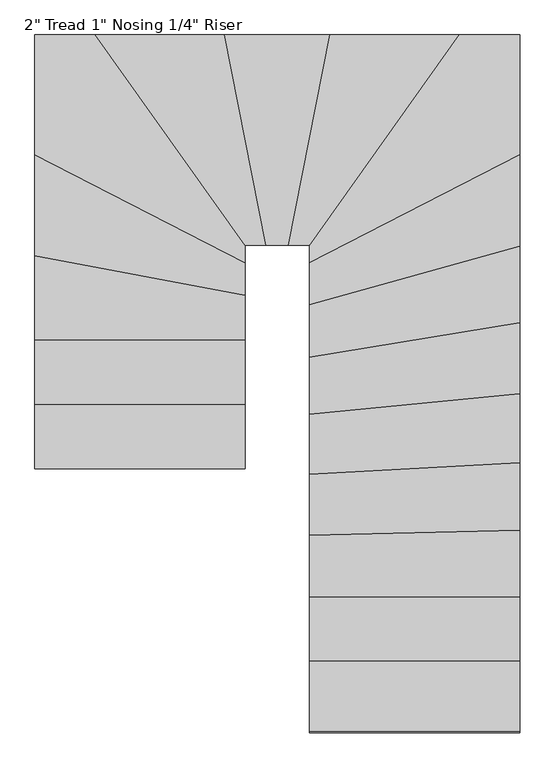
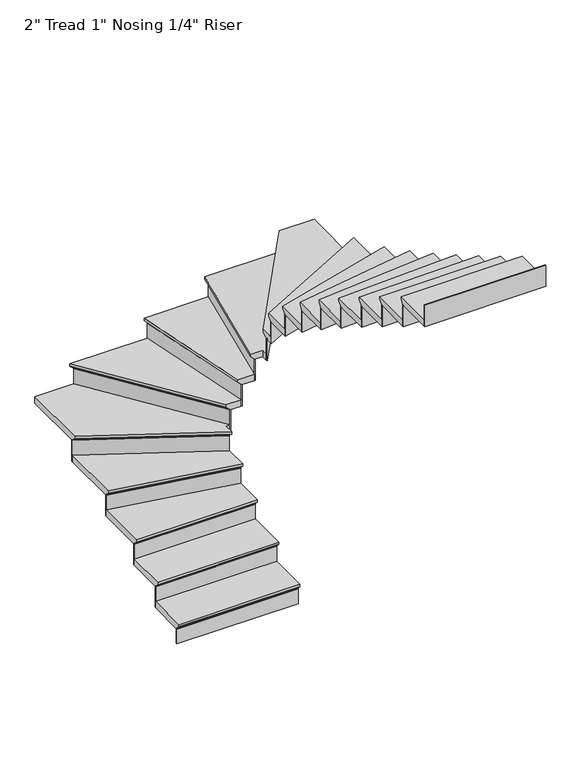
"""IFC4 building model written with IfcOpenShell, lengths in millimetres: stair flight geometry."""

from ifc_helpers import new_model, si_unit, origin, place, context, project, spatial, faceted_brep, source, transform, mapped, element, save


def stair_flight_4b05d3ae(model_context):
    return source(origin(), model_context, "Body", "Brep", [
        faceted_brep([(-9210.4744419, 9071.9135491, 488.95), (-9210.4744419, 9071.9135491, 508.0), (-10124.8744419, 9071.9135491, 508.0), (-10124.8744419, 9071.9135491, 488.95), (-9210.4744419, 9097.3135491, 463.55), (-10124.8744419, 9097.3135491, 463.55), (-9210.4744419, 9376.7135491, 508.0), (-10124.8744419, 9376.7135491, 508.0), (-10124.8744419, 9097.3135491, 457.2), (-10124.8744419, 9376.7135491, 457.2), (-9210.4744419, 9376.7135491, 457.2), (-9210.4744419, 9097.3135491, 457.2)], [[[0, 1, 2, 3]], [[4, 0, 3, 5]], [[2, 1, 6, 7]], [[8, 9, 10, 11]], [[2, 7, 9, 8, 5, 3]], [[8, 11, 4, 5]], [[6, 1, 0, 4, 11, 10]], [[7, 6, 10, 9]]]),
        faceted_brep([(-9210.4744419, 9097.3135491, 457.2), (-9210.4744419, 9097.3135491, 338.6666667), (-9210.4744419, 9103.6635491, 338.6666667), (-9210.4744419, 9103.6635491, 457.2), (-10124.8744419, 9097.3135491, 457.2), (-10124.8744419, 9103.6635491, 457.2), (-10124.8744419, 9103.6635491, 338.6666667), (-10124.8744419, 9097.3135491, 338.6666667)], [[[0, 1, 2, 3]], [[4, 5, 6, 7]], [[1, 0, 4, 7]], [[2, 1, 7, 6]], [[3, 2, 6, 5]], [[0, 3, 5, 4]]]),
        faceted_brep([(-9210.4744419, 9376.7135491, 626.5333333), (-9210.4744419, 9376.7135491, 457.2), (-9210.4744419, 9383.0635491, 457.2), (-9210.4744419, 9383.0635491, 626.5333333), (-10124.8744419, 9376.7135491, 626.5333333), (-10124.8744419, 9383.0635491, 626.5333333), (-10124.8744419, 9383.0635491, 457.2), (-10124.8744419, 9376.7135491, 457.2)], [[[0, 1, 2, 3]], [[4, 5, 6, 7]], [[1, 0, 4, 7]], [[2, 1, 7, 6]], [[3, 2, 6, 5]], [[0, 3, 5, 4]]]),
        faceted_brep([(-10124.8744419, 9351.3135491, 677.3333333), (-9210.4744419, 9351.3135491, 677.3333333), (-9210.4744419, 9656.1135491, 677.3333333), (-10124.8744419, 9656.1135491, 677.3333333), (-10124.8744419, 9376.7135491, 626.5333333), (-10124.8744419, 9656.1135491, 626.5333333), (-9210.4744419, 9656.1135491, 626.5333333), (-9210.4744419, 9376.7135491, 626.5333333), (-10124.8744419, 9376.7135491, 632.8833333), (-10124.8744419, 9351.3135491, 658.2833333), (-9210.4744419, 9376.7135491, 632.8833333), (-9210.4744419, 9351.3135491, 658.2833333)], [[[0, 1, 2, 3]], [[4, 5, 6, 7]], [[0, 3, 5, 4, 8, 9]], [[4, 7, 10, 8]], [[2, 1, 11, 10, 7, 6]], [[3, 2, 6, 5]], [[11, 1, 0, 9]], [[10, 11, 9, 8]]]),
        faceted_brep([(-9210.4744419, 9656.1135491, 795.8666667), (-9210.4744419, 9656.1135491, 626.5333333), (-9210.4744419, 9662.4635491, 626.5333333), (-9210.4744419, 9662.4635491, 795.8666667), (-10124.8744419, 9656.1135491, 795.8666667), (-10124.8744419, 9662.4635491, 795.8666667), (-10124.8744419, 9662.4635491, 626.5333333), (-10124.8744419, 9656.1135491, 626.5333333)], [[[0, 1, 2, 3]], [[4, 5, 6, 7]], [[1, 0, 4, 7]], [[2, 1, 7, 6]], [[3, 2, 6, 5]], [[0, 3, 5, 4]]]),
        faceted_brep([(-10124.8744419, 9630.7135491, 846.6666667), (-9210.4744419, 9630.7135491, 846.6666667), (-9210.4744419, 9849.4936887, 846.6666667), (-10124.8744419, 10022.433987, 846.6666667), (-10124.8744419, 9656.1135491, 795.8666667), (-10124.8744419, 10022.433987, 795.8666667), (-9210.4744419, 9849.4936887, 795.8666667), (-9210.4744419, 9656.1135491, 795.8666667), (-10124.8744419, 9656.1135491, 802.2166667), (-10124.8744419, 9630.7135491, 827.6166667), (-9210.4744419, 9656.1135491, 802.2166667), (-9210.4744419, 9630.7135491, 827.6166667)], [[[0, 1, 2, 3]], [[4, 5, 6, 7]], [[0, 3, 5, 4, 8, 9]], [[4, 7, 10, 8]], [[2, 1, 11, 10, 7, 6]], [[3, 2, 6, 5]], [[11, 1, 0, 9]], [[10, 11, 9, 8]]]),
        faceted_brep([(-9210.4744419, 9849.4936887, 965.2), (-9210.4744419, 9849.4936887, 795.8666667), (-9210.4744419, 9855.9562608, 795.8666667), (-9210.4744419, 9855.9562608, 965.2), (-10124.8744419, 10022.433987, 965.2), (-10124.8744419, 10028.8965592, 965.2), (-10124.8744419, 10028.8965592, 795.8666667), (-10124.8744419, 10022.433987, 795.8666667)], [[[0, 1, 2, 3]], [[4, 5, 6, 7]], [[1, 0, 4, 7]], [[2, 1, 7, 6]], [[3, 2, 6, 5]], [[0, 3, 5, 4]]]),
        faceted_brep([(-10124.8744419, 9996.5836983, 1016.0), (-9210.4744419, 9823.6433999, 1016.0), (-9210.4744419, 9995.1212689, 1016.0), (-10124.8744419, 10463.9458903, 1016.0), (-10124.8744419, 10022.433987, 965.2), (-10124.8744419, 10463.9458903, 965.2), (-9210.4744419, 9995.1212689, 965.2), (-9210.4744419, 9849.4936887, 965.2), (-10124.8744419, 10022.433987, 971.55), (-10124.8744419, 9996.5836983, 996.95), (-9210.4744419, 9849.4936887, 971.55), (-9210.4744419, 9823.6433999, 996.95)], [[[0, 1, 2, 3]], [[4, 5, 6, 7]], [[0, 3, 5, 4, 8, 9]], [[4, 7, 10, 8]], [[2, 1, 11, 10, 7, 6]], [[3, 2, 6, 5]], [[11, 1, 0, 9]], [[10, 11, 9, 8]]]),
        faceted_brep([(-9210.4744419, 9995.1212689, 1134.5333333), (-9210.4744419, 9995.1212689, 965.2), (-9210.4744419, 10002.2572521, 965.2), (-9210.4744419, 10002.2572521, 1134.5333333), (-10124.8744419, 10463.9458903, 1134.5333333), (-10124.8744419, 10471.0818734, 1134.5333333), (-10124.8744419, 10471.0818734, 965.2), (-10124.8744419, 10463.9458903, 965.2)], [[[0, 1, 2, 3]], [[4, 5, 6, 7]], [[1, 0, 4, 7]], [[2, 1, 7, 6]], [[3, 2, 6, 5]], [[0, 3, 5, 4]]]),
        faceted_brep([(-9831.1933082, 10955.2452409, 1185.3333333), (-10124.8744419, 10955.2452409, 1185.3333333), (-10124.8744419, 10435.4019577, 1185.3333333), (-9210.4744419, 9966.5773364, 1185.3333333), (-9210.4744419, 10040.8452409, 1185.3333333), (-9180.9193591, 10040.8452409, 1185.3333333), (-10124.8744419, 10955.2452409, 1134.5333333), (-9831.1933082, 10955.2452409, 1134.5333333), (-9180.9193591, 10040.8452409, 1134.5333333), (-9210.4744419, 10040.8452409, 1134.5333333), (-9210.4744419, 9995.1212689, 1134.5333333), (-10124.8744419, 10463.9458903, 1134.5333333), (-9210.4744419, 9995.1212689, 1140.8833333), (-10124.8744419, 10463.9458903, 1140.8833333), (-9210.4744419, 9966.5773364, 1166.2833333), (-10124.8744419, 10435.4019577, 1166.2833333)], [[[0, 1, 2, 3, 4, 5]], [[6, 7, 8, 9, 10, 11]], [[1, 0, 7, 6]], [[11, 10, 12, 13]], [[4, 3, 14, 12, 10, 9]], [[0, 5, 8, 7]], [[14, 3, 2, 15]], [[12, 14, 15, 13]], [[2, 1, 6, 11, 13, 15]], [[5, 4, 9, 8]]]),
        faceted_brep([(-9180.9193591, 10040.8452409, 1303.8666667), (-9180.9193591, 10040.8452409, 1134.5333333), (-9173.1273843, 10040.8452409, 1134.5333333), (-9173.1273843, 10040.8452409, 1303.8666667), (-9831.1933082, 10955.2452409, 1303.8666667), (-9823.4013334, 10955.2452409, 1303.8666667), (-9823.4013334, 10955.2452409, 1134.5333333), (-9831.1933082, 10955.2452409, 1134.5333333)], [[[0, 1, 2, 3]], [[4, 5, 6, 7]], [[1, 0, 4, 7]], [[2, 1, 7, 6]], [[3, 2, 6, 5]], [[0, 3, 5, 4]]]),
        faceted_brep([(-9862.3612074, 10955.2452409, 1354.6666667), (-9212.0872582, 10040.8452409, 1354.6666667), (-9094.465272, 10040.8452409, 1354.6666667), (-9274.7061283, 10955.2452409, 1354.6666667), (-9831.1933082, 10955.2452409, 1303.8666667), (-9274.7061283, 10955.2452409, 1303.8666667), (-9094.465272, 10040.8452409, 1303.8666667), (-9180.9193591, 10040.8452409, 1303.8666667), (-9831.1933082, 10955.2452409, 1310.2166667), (-9862.3612074, 10955.2452409, 1335.6166667), (-9180.9193591, 10040.8452409, 1310.2166667), (-9212.0872582, 10040.8452409, 1335.6166667)], [[[0, 1, 2, 3]], [[4, 5, 6, 7]], [[0, 3, 5, 4, 8, 9]], [[4, 7, 10, 8]], [[3, 2, 6, 5]], [[11, 1, 0, 9]], [[10, 11, 9, 8]], [[2, 1, 11, 10, 7, 6]]]),
        faceted_brep([(-9094.465272, 10040.8452409, 1473.2), (-9094.465272, 10040.8452409, 1303.8666667), (-9087.9930866, 10040.8452409, 1303.8666667), (-9087.9930866, 10040.8452409, 1473.2), (-9274.7061283, 10955.2452409, 1473.2), (-9268.2339429, 10955.2452409, 1473.2), (-9268.2339429, 10955.2452409, 1303.8666667), (-9274.7061283, 10955.2452409, 1303.8666667)], [[[0, 1, 2, 3]], [[4, 5, 6, 7]], [[1, 0, 4, 7]], [[2, 1, 7, 6]], [[3, 2, 6, 5]], [[0, 3, 5, 4]]]),
        faceted_brep([(-9300.5948701, 10955.2452409, 1524.0), (-9120.3540137, 10040.8452409, 1524.0), (-8995.3061283, 10040.8452409, 1524.0), (-8815.065272, 10955.2452409, 1524.0), (-9274.7061283, 10955.2452409, 1473.2), (-8815.065272, 10955.2452409, 1473.2), (-8995.3061283, 10040.8452409, 1473.2), (-9094.465272, 10040.8452409, 1473.2), (-9274.7061283, 10955.2452409, 1479.55), (-9300.5948701, 10955.2452409, 1504.95), (-9094.465272, 10040.8452409, 1479.55), (-9120.3540137, 10040.8452409, 1504.95)], [[[0, 1, 2, 3]], [[4, 5, 6, 7]], [[0, 3, 5, 4, 8, 9]], [[4, 7, 10, 8]], [[2, 1, 11, 10, 7, 6]], [[3, 2, 6, 5]], [[11, 1, 0, 9]], [[10, 11, 9, 8]]]),
        faceted_brep([(-8995.3061283, 10040.8452409, 1642.5333333), (-8995.3061283, 10040.8452409, 1473.2), (-8988.8339429, 10040.8452409, 1473.2), (-8988.8339429, 10040.8452409, 1642.5333333), (-8815.065272, 10955.2452409, 1642.5333333), (-8808.5930866, 10955.2452409, 1642.5333333), (-8808.5930866, 10955.2452409, 1473.2), (-8815.065272, 10955.2452409, 1473.2)], [[[0, 1, 2, 3]], [[4, 5, 6, 7]], [[1, 0, 4, 7]], [[2, 1, 7, 6]], [[3, 2, 6, 5]], [[0, 3, 5, 4]]]),
        faceted_brep([(-8840.9540137, 10955.2452409, 1693.3333333), (-9021.1948701, 10040.8452409, 1693.3333333), (-8931.0744419, 10040.8452409, 1693.3333333), (-8931.0744419, 9994.7497664, 1693.3333333), (-8248.0197772, 10955.2452409, 1693.3333333), (-8815.065272, 10955.2452409, 1642.5333333), (-8248.0197772, 10955.2452409, 1642.5333333), (-8931.0744419, 9994.7497664, 1642.5333333), (-8931.0744419, 10040.8452409, 1642.5333333), (-8995.3061283, 10040.8452409, 1642.5333333), (-8815.065272, 10955.2452409, 1648.8833333), (-8840.9540137, 10955.2452409, 1674.2833333), (-8995.3061283, 10040.8452409, 1648.8833333), (-9021.1948701, 10040.8452409, 1674.2833333)], [[[0, 1, 2, 3, 4]], [[5, 6, 7, 8, 9]], [[0, 4, 6, 5, 10, 11]], [[5, 9, 12, 10]], [[3, 2, 8, 7]], [[4, 3, 7, 6]], [[13, 1, 0, 11]], [[12, 13, 11, 10]], [[2, 1, 13, 12, 9, 8]]]),
        faceted_brep([(-8931.0744419, 9994.7497664, 1811.8666667), (-8931.0744419, 9994.7497664, 1642.5333333), (-8931.0744419, 9983.7928739, 1642.5333333), (-8931.0744419, 9983.7928739, 1811.8666667), (-8248.0197772, 10955.2452409, 1811.8666667), (-8240.2278025, 10955.2452409, 1811.8666667), (-8240.2278025, 10955.2452409, 1642.5333333), (-8248.0197772, 10955.2452409, 1642.5333333)], [[[0, 1, 2, 3]], [[4, 5, 6, 7]], [[1, 0, 4, 7]], [[2, 1, 7, 6]], [[3, 2, 6, 5]], [[0, 3, 5, 4]]]),
        faceted_brep([(-8016.6744419, 10406.8580252, 1862.6666667), (-8016.6744419, 10955.2452409, 1862.6666667), (-8279.1876764, 10955.2452409, 1862.6666667), (-8931.0744419, 10038.5773364, 1862.6666667), (-8931.0744419, 9938.0334039, 1862.6666667), (-8016.6744419, 10955.2452409, 1811.8666667), (-8016.6744419, 10406.8580252, 1811.8666667), (-8931.0744419, 9938.0334039, 1811.8666667), (-8931.0744419, 9994.7497664, 1811.8666667), (-8248.0197772, 10955.2452409, 1811.8666667), (-8931.0744419, 9994.7497664, 1818.2166667), (-8248.0197772, 10955.2452409, 1818.2166667), (-8931.0744419, 10038.5773364, 1843.6166667), (-8279.1876764, 10955.2452409, 1843.6166667)], [[[0, 1, 2, 3, 4]], [[5, 6, 7, 8, 9]], [[1, 0, 6, 5]], [[9, 8, 10, 11]], [[4, 3, 12, 10, 8, 7]], [[0, 4, 7, 6]], [[12, 3, 2, 13]], [[10, 12, 13, 11]], [[2, 1, 5, 9, 11, 13]]]),
        faceted_brep([(-8931.0744419, 9938.0334039, 1981.2), (-8931.0744419, 9938.0334039, 1811.8666667), (-8931.0744419, 9930.8974207, 1811.8666667), (-8931.0744419, 9930.8974207, 1981.2), (-8016.6744419, 10406.8580252, 1981.2), (-8016.6744419, 10399.7220421, 1981.2), (-8016.6744419, 10399.7220421, 1811.8666667), (-8016.6744419, 10406.8580252, 1811.8666667)], [[[0, 1, 2, 3]], [[4, 5, 6, 7]], [[1, 0, 4, 7]], [[2, 1, 7, 6]], [[3, 2, 6, 5]], [[0, 3, 5, 4]]]),
        faceted_brep([(-8016.6744419, 10435.4019577, 2032.0), (-8931.0744419, 9966.5773364, 2032.0), (-8931.0744419, 9757.0807596, 2032.0), (-8016.6744419, 10010.432504, 2032.0), (-8016.6744419, 10406.8580252, 1981.2), (-8016.6744419, 10010.432504, 1981.2), (-8931.0744419, 9757.0807596, 1981.2), (-8931.0744419, 9938.0334039, 1981.2), (-8016.6744419, 10406.8580252, 1987.55), (-8016.6744419, 10435.4019577, 2012.95), (-8931.0744419, 9938.0334039, 1987.55), (-8931.0744419, 9966.5773364, 2012.95)], [[[0, 1, 2, 3]], [[4, 5, 6, 7]], [[0, 3, 5, 4, 8, 9]], [[4, 7, 10, 8]], [[2, 1, 11, 10, 7, 6]], [[3, 2, 6, 5]], [[11, 1, 0, 9]], [[10, 11, 9, 8]]]),
        faceted_brep([(-8931.0744419, 9757.0807596, 2150.5333333), (-8931.0744419, 9757.0807596, 1981.2), (-8931.0744419, 9750.4915303, 1981.2), (-8931.0744419, 9750.4915303, 2150.5333333), (-8016.6744419, 10010.432504, 2150.5333333), (-8016.6744419, 10003.8432747, 2150.5333333), (-8016.6744419, 10003.8432747, 1981.2), (-8016.6744419, 10010.432504, 1981.2)], [[[0, 1, 2, 3]], [[4, 5, 6, 7]], [[1, 0, 4, 7]], [[2, 1, 7, 6]], [[3, 2, 6, 5]], [[0, 3, 5, 4]]]),
        faceted_brep([(-8016.6744419, 10036.7894213, 2201.3333333), (-8931.0744419, 9783.4376768, 2201.3333333), (-8931.0744419, 9529.7422871, 2201.3333333), (-8016.6744419, 9680.2017024, 2201.3333333), (-8016.6744419, 10010.432504, 2150.5333333), (-8016.6744419, 9680.2017024, 2150.5333333), (-8931.0744419, 9529.7422871, 2150.5333333), (-8931.0744419, 9757.0807596, 2150.5333333), (-8016.6744419, 10010.432504, 2156.8833333), (-8016.6744419, 10036.7894213, 2182.2833333), (-8931.0744419, 9757.0807596, 2156.8833333), (-8931.0744419, 9783.4376768, 2182.2833333)], [[[0, 1, 2, 3]], [[4, 5, 6, 7]], [[0, 3, 5, 4, 8, 9]], [[4, 7, 10, 8]], [[2, 1, 11, 10, 7, 6]], [[3, 2, 6, 5]], [[11, 1, 0, 9]], [[10, 11, 9, 8]]]),
        faceted_brep([(-8931.0744419, 9529.7422871, 2319.8666667), (-8931.0744419, 9529.7422871, 2150.5333333), (-8931.0744419, 9523.3068985, 2150.5333333), (-8931.0744419, 9523.3068985, 2319.8666667), (-8016.6744419, 9680.2017024, 2319.8666667), (-8016.6744419, 9673.7663138, 2319.8666667), (-8016.6744419, 9673.7663138, 2150.5333333), (-8016.6744419, 9680.2017024, 2150.5333333)], [[[0, 1, 2, 3]], [[4, 5, 6, 7]], [[1, 0, 4, 7]], [[2, 1, 7, 6]], [[3, 2, 6, 5]], [[0, 3, 5, 4]]]),
        faceted_brep([(-8016.6744419, 9705.9432567, 2370.6666667), (-8931.0744419, 9555.4838414, 2370.6666667), (-8931.0744419, 9280.9284936, 2370.6666667), (-8016.6744419, 9370.6546227, 2370.6666667), (-8016.6744419, 9680.2017024, 2319.8666667), (-8016.6744419, 9370.6546227, 2319.8666667), (-8931.0744419, 9280.9284936, 2319.8666667), (-8931.0744419, 9529.7422871, 2319.8666667), (-8016.6744419, 9680.2017024, 2326.2166667), (-8016.6744419, 9705.9432567, 2351.6166667), (-8931.0744419, 9529.7422871, 2326.2166667), (-8931.0744419, 9555.4838414, 2351.6166667)], [[[0, 1, 2, 3]], [[4, 5, 6, 7]], [[0, 3, 5, 4, 8, 9]], [[4, 7, 10, 8]], [[2, 1, 11, 10, 7, 6]], [[3, 2, 6, 5]], [[11, 1, 0, 9]], [[10, 11, 9, 8]]]),
        faceted_brep([(-8931.0744419, 9280.9284936, 2489.2), (-8931.0744419, 9280.9284936, 2319.8666667), (-8931.0744419, 9274.5479959, 2319.8666667), (-8931.0744419, 9274.5479959, 2489.2), (-8016.6744419, 9370.6546227, 2489.2), (-8016.6744419, 9364.274125, 2489.2), (-8016.6744419, 9364.274125, 2319.8666667), (-8016.6744419, 9370.6546227, 2319.8666667)], [[[0, 1, 2, 3]], [[4, 5, 6, 7]], [[1, 0, 4, 7]], [[2, 1, 7, 6]], [[3, 2, 6, 5]], [[0, 3, 5, 4]]]),
        faceted_brep([(-8016.6744419, 9396.1766136, 2540.0), (-8931.0744419, 9306.4504846, 2540.0), (-8931.0744419, 9021.6529492, 2540.0), (-8016.6744419, 9071.2993292, 2540.0), (-8016.6744419, 9370.6546227, 2489.2), (-8016.6744419, 9071.2993292, 2489.2), (-8931.0744419, 9021.6529492, 2489.2), (-8931.0744419, 9280.9284936, 2489.2), (-8016.6744419, 9370.6546227, 2495.55), (-8016.6744419, 9396.1766136, 2520.95), (-8931.0744419, 9280.9284936, 2495.55), (-8931.0744419, 9306.4504846, 2520.95)], [[[0, 1, 2, 3]], [[4, 5, 6, 7]], [[0, 3, 5, 4, 8, 9]], [[4, 7, 10, 8]], [[2, 1, 11, 10, 7, 6]], [[3, 2, 6, 5]], [[11, 1, 0, 9]], [[10, 11, 9, 8]]]),
        faceted_brep([(-8931.0744419, 9021.6529492, 2658.5333333), (-8931.0744419, 9021.6529492, 2489.2), (-8931.0744419, 9015.2935967, 2489.2), (-8931.0744419, 9015.2935967, 2658.5333333), (-8016.6744419, 9071.2993292, 2658.5333333), (-8016.6744419, 9064.9399767, 2658.5333333), (-8016.6744419, 9064.9399767, 2489.2), (-8016.6744419, 9071.2993292, 2489.2)], [[[0, 1, 2, 3]], [[4, 5, 6, 7]], [[1, 0, 4, 7]], [[2, 1, 7, 6]], [[3, 2, 6, 5]], [[0, 3, 5, 4]]]),
        faceted_brep([(-8016.6744419, 9096.7367391, 2709.3333333), (-8931.0744419, 9047.0903591, 2709.3333333), (-8931.0744419, 8756.4988274, 2709.3333333), (-8016.6744419, 8777.7145991, 2709.3333333), (-8016.6744419, 9071.2993292, 2658.5333333), (-8016.6744419, 8777.7145991, 2658.5333333), (-8931.0744419, 8756.4988274, 2658.5333333), (-8931.0744419, 9021.6529492, 2658.5333333), (-8016.6744419, 9071.2993292, 2664.8833333), (-8016.6744419, 9096.7367391, 2690.2833333), (-8931.0744419, 9021.6529492, 2664.8833333), (-8931.0744419, 9047.0903591, 2690.2833333)], [[[0, 1, 2, 3]], [[4, 5, 6, 7]], [[0, 3, 5, 4, 8, 9]], [[4, 7, 10, 8]], [[2, 1, 11, 10, 7, 6]], [[3, 2, 6, 5]], [[11, 1, 0, 9]], [[10, 11, 9, 8]]]),
        faceted_brep([(-8931.0744419, 8756.4988274, 2827.8666667), (-8931.0744419, 8756.4988274, 2658.5333333), (-8931.0744419, 8750.1471184, 2658.5333333), (-8931.0744419, 8750.1471184, 2827.8666667), (-8016.6744419, 8777.7145991, 2827.8666667), (-8016.6744419, 8771.3628902, 2827.8666667), (-8016.6744419, 8771.3628902, 2658.5333333), (-8016.6744419, 8777.7145991, 2658.5333333)], [[[0, 1, 2, 3]], [[4, 5, 6, 7]], [[1, 0, 4, 7]], [[2, 1, 7, 6]], [[3, 2, 6, 5]], [[0, 3, 5, 4]]]),
        faceted_brep([(-8016.6744419, 8803.121435, 2878.6666667), (-8931.0744419, 8781.9056632, 2878.6666667), (-8931.0744419, 8487.7135491, 2878.6666667), (-8016.6744419, 8487.7135491, 2878.6666667), (-8016.6744419, 8777.7145991, 2827.8666667), (-8016.6744419, 8487.7135491, 2827.8666667), (-8931.0744419, 8487.7135491, 2827.8666667), (-8931.0744419, 8756.4988274, 2827.8666667), (-8016.6744419, 8777.7145991, 2834.2166667), (-8016.6744419, 8803.121435, 2859.6166667), (-8931.0744419, 8756.4988274, 2834.2166667), (-8931.0744419, 8781.9056632, 2859.6166667)], [[[0, 1, 2, 3]], [[4, 5, 6, 7]], [[0, 3, 5, 4, 8, 9]], [[4, 7, 10, 8]], [[2, 1, 11, 10, 7, 6]], [[3, 2, 6, 5]], [[11, 1, 0, 9]], [[10, 11, 9, 8]]]),
        faceted_brep([(-8931.0744419, 8487.7135491, 2997.2), (-8931.0744419, 8487.7135491, 2827.8666667), (-8931.0744419, 8481.3635491, 2827.8666667), (-8931.0744419, 8481.3635491, 2997.2), (-8016.6744419, 8487.7135491, 2997.2), (-8016.6744419, 8481.3635491, 2997.2), (-8016.6744419, 8481.3635491, 2827.8666667), (-8016.6744419, 8487.7135491, 2827.8666667)], [[[0, 1, 2, 3]], [[4, 5, 6, 7]], [[1, 0, 4, 7]], [[2, 1, 7, 6]], [[3, 2, 6, 5]], [[0, 3, 5, 4]]]),
        faceted_brep([(-8016.6744419, 8513.1135491, 3048.0), (-8931.0744419, 8513.1135491, 3048.0), (-8931.0744419, 8208.3135491, 3048.0), (-8016.6744419, 8208.3135491, 3048.0), (-8016.6744419, 8487.7135491, 2997.2), (-8016.6744419, 8208.3135491, 2997.2), (-8931.0744419, 8208.3135491, 2997.2), (-8931.0744419, 8487.7135491, 2997.2), (-8016.6744419, 8487.7135491, 3003.55), (-8016.6744419, 8513.1135491, 3028.95), (-8931.0744419, 8487.7135491, 3003.55), (-8931.0744419, 8513.1135491, 3028.95)], [[[0, 1, 2, 3]], [[4, 5, 6, 7]], [[0, 3, 5, 4, 8, 9]], [[4, 7, 10, 8]], [[2, 1, 11, 10, 7, 6]], [[3, 2, 6, 5]], [[11, 1, 0, 9]], [[10, 11, 9, 8]]]),
        faceted_brep([(-8931.0744419, 8208.3135491, 3166.5333333), (-8931.0744419, 8208.3135491, 2997.2), (-8931.0744419, 8201.9635491, 2997.2), (-8931.0744419, 8201.9635491, 3166.5333333), (-8016.6744419, 8208.3135491, 3166.5333333), (-8016.6744419, 8201.9635491, 3166.5333333), (-8016.6744419, 8201.9635491, 2997.2), (-8016.6744419, 8208.3135491, 2997.2)], [[[0, 1, 2, 3]], [[4, 5, 6, 7]], [[1, 0, 4, 7]], [[2, 1, 7, 6]], [[3, 2, 6, 5]], [[0, 3, 5, 4]]]),
        faceted_brep([(-8931.0744419, 7928.9135491, 3335.8666667), (-8931.0744419, 7928.9135491, 3166.5333333), (-8931.0744419, 7922.5635491, 3166.5333333), (-8931.0744419, 7922.5635491, 3335.8666667), (-8016.6744419, 7928.9135491, 3335.8666667), (-8016.6744419, 7922.5635491, 3335.8666667), (-8016.6744419, 7922.5635491, 3166.5333333), (-8016.6744419, 7928.9135491, 3166.5333333)], [[[0, 1, 2, 3]], [[4, 5, 6, 7]], [[1, 0, 4, 7]], [[2, 1, 7, 6]], [[3, 2, 6, 5]], [[0, 3, 5, 4]]]),
        faceted_brep([(-8016.6744419, 8233.7135491, 3217.3333333), (-8931.0744419, 8233.7135491, 3217.3333333), (-8931.0744419, 7928.9135491, 3217.3333333), (-8016.6744419, 7928.9135491, 3217.3333333), (-8016.6744419, 8208.3135491, 3166.5333333), (-8016.6744419, 7928.9135491, 3166.5333333), (-8931.0744419, 7928.9135491, 3166.5333333), (-8931.0744419, 8208.3135491, 3166.5333333), (-8016.6744419, 8208.3135491, 3172.8833333), (-8016.6744419, 8233.7135491, 3198.2833333), (-8931.0744419, 8208.3135491, 3172.8833333), (-8931.0744419, 8233.7135491, 3198.2833333)], [[[0, 1, 2, 3]], [[4, 5, 6, 7]], [[0, 3, 5, 4, 8, 9]], [[4, 7, 10, 8]], [[2, 1, 11, 10, 7, 6]], [[3, 2, 6, 5]], [[11, 1, 0, 9]], [[10, 11, 9, 8]]]),
    ])


if __name__ == "__main__":
    model = new_model("IFC4")
    model_context = context("Model", 3, world=origin())
    ifc_project = project(units=[si_unit("LENGTHUNIT", "METRE", prefix="MILLI")], contexts=[model_context])
    site = spatial("IfcSite", under=ifc_project)
    building = spatial("IfcBuilding", under=site)
    placement = place(None, origin())
    stair_flight_shape = stair_flight_4b05d3ae(model_context)
    element("IfcStairFlight", 1, ObjectType="2\" Tread 1\" Nosing 1/4\" Riser", at=placement, inside=building, context=model_context, shape_type="MappedRepresentation", body=[
        mapped(stair_flight_shape, transform((0.0, 0.0, 0.0), x_axis=(1.0, 0.0, 0.0), y_axis=(0.0, 1.0, 0.0), z_axis=(0.0, 0.0, 1.0))),
    ])
    save(model, "model.ifc")
